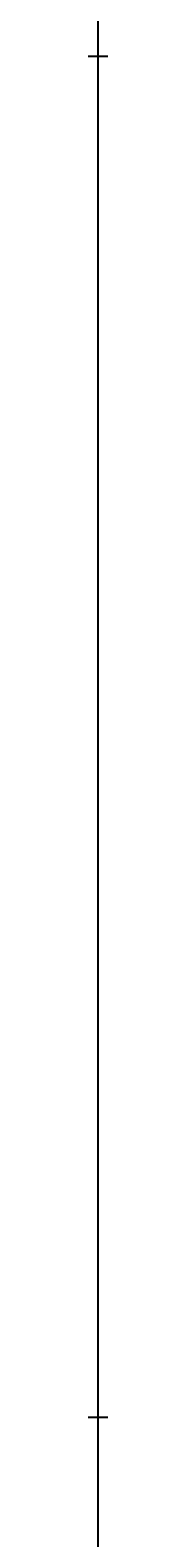
# Model space of a CAD drawing. Units: inches. Extents: x 35362 to 73946, y 43607 to 67532.
# Tile 38 of 134: x 48373 to 48373, y 46091 to 46564. Entities that reach past the tile are written whole.
import ezdxf

# ---------------------------------------------------------------- set-up
doc = ezdxf.new("R2010")
doc.units = ezdxf.units.IN
doc.header["$MEASUREMENT"] = 0
doc.layers.add('A-ANNO-DIMS', color=2, linetype='Continuous', lineweight=18)
doc.styles.get("Standard").update_dxf_attribs({"font": 'arial.ttf'})
doc.dimstyles.get("Standard").update_dxf_attribs({"dimtxt": 0.18, "dimasz": 0.18, "dimexe": 0.18, "dimexo": 0.0625, "dimgap": 0.09, "dimtad": 0, "dimtih": 1, "dimtoh": 1, "dimdec": 4, "dimzin": 0, "dimdsep": 46, "dimtxsty": 'Standard', "dimcen": 0.09, "dimadec": 0, "dimazin": 0, "dimtfac": 1, "dimtdec": 4, "dimtofl": 0, "dimtmove": 0, "dimatfit": 3, "dimfxl": 1, "dimtolj": 1, "dimtzin": 0, "dimarcsym": 0})

# ---------------------------------------------------------------- blocks, each defined once
blk = doc.blocks.new('*D5')
at = {"layer": 'A-ANNO-DIMS', "color": 0, "lineweight": -2, "transparency": 16777216}
for p, q in [((37121.95, 46919.32), (37121.95, 43606.68)), ((69871.5, 45449.83), (69871.5, 43606.68)), ((37122.13, 43606.86), (53496.29, 43606.86)), ((69871.32, 43606.86), (53497.15, 43606.86))]:
    blk.add_line(p, q, dxfattribs=at)
at = {"layer": 'A-ANNO-DIMS', "color": 0, "transparency": 16777216}
for points in [[(37122.13, 43606.89), (37122.13, 43606.83), (37121.95, 43606.86)], [(69871.32, 43606.89), (69871.32, 43606.83), (69871.5, 43606.86)]]:
    blk.add_solid(points, dxfattribs=at)
at = {"layer": 'Defpoints', "color": 0, "transparency": 16777216}
for p in [(37121.95, 46919.38), (69871.5, 45449.89), (69871.5, 43606.86)]:
    blk.add_point(p, dxfattribs=at)
at = {"layer": 'A-ANNO-DIMS', "color": 0, "transparency": 16777216, "insert": (53496.72, 43606.86), "char_height": 0.18, "attachment_point": 5}
blk.add_mtext('\\A1;32750', dxfattribs=at)
blk = doc.blocks.new('*D11')
at = {"layer": 'A-ANNO-DIMS', "color": 0, "lineweight": -2, "transparency": 16777216}
for p, q in [((47978.66, 56028.77), (47978.66, 43606.68)), ((53109.76, 56028.77), (53109.76, 43606.68)), ((47978.84, 43606.86), (50543.87, 43606.86)), ((53109.58, 43606.86), (50544.55, 43606.86))]:
    blk.add_line(p, q, dxfattribs=at)
at = {"layer": 'A-ANNO-DIMS', "color": 0, "transparency": 16777216}
for points in [[(47978.84, 43606.89), (47978.84, 43606.83), (47978.66, 43606.86)], [(53109.58, 43606.89), (53109.58, 43606.83), (53109.76, 43606.86)]]:
    blk.add_solid(points, dxfattribs=at)
at = {"layer": 'Defpoints', "color": 0, "transparency": 16777216}
for p in [(47978.66, 56028.84), (53109.76, 56028.84), (53109.76, 43606.86)]:
    blk.add_point(p, dxfattribs=at)
at = {"layer": 'A-ANNO-DIMS', "color": 0, "transparency": 16777216, "insert": (50544.21, 43606.86), "char_height": 0.18, "attachment_point": 5}
blk.add_mtext('\\A1;5131', dxfattribs=at)
blk = doc.blocks.new('*D13')
at = {"layer": 'A-ANNO-DIMS', "color": 0, "lineweight": -2, "transparency": 16777216}
for p, q in [((48373.49, 51694.02), (48373.49, 43606.68)), ((51029.04, 51694.02), (51029.04, 43606.68)), ((48373.67, 43606.86), (49700.8, 43606.86)), ((51028.86, 43606.86), (49701.73, 43606.86))]:
    blk.add_line(p, q, dxfattribs=at)
at = {"layer": 'A-ANNO-DIMS', "color": 0, "transparency": 16777216}
for points in [[(48373.67, 43606.89), (48373.67, 43606.83), (48373.49, 43606.86)], [(51028.86, 43606.89), (51028.86, 43606.83), (51029.04, 43606.86)]]:
    blk.add_solid(points, dxfattribs=at)
at = {"layer": 'Defpoints', "color": 0, "transparency": 16777216}
for p in [(48373.49, 51694.09), (51029.04, 51694.09), (51029.04, 43606.86)]:
    blk.add_point(p, dxfattribs=at)
at = {"layer": 'A-ANNO-DIMS', "color": 0, "transparency": 16777216, "insert": (49701.27, 43606.86), "char_height": 0.18, "attachment_point": 5}
blk.add_mtext('\\A1;2655.6', dxfattribs=at)
blk = doc.blocks.new('*D67')
at = {"layer": 'A-ANNO-DIMS', "color": 0, "lineweight": -2, "transparency": 16777216}
for p, q in [((56873.54, 53351.53), (35361.77, 53351.53)), ((35361.95, 53351.35), (35361.95, 49400.89)), ((35361.95, 45450.07), (35361.95, 49400.53)), ((53793.58, 45449.89), (35361.77, 45449.89))]:
    blk.add_line(p, q, dxfattribs=at)
at = {"layer": 'A-ANNO-DIMS', "color": 0, "transparency": 16777216}
for points in [[(35361.92, 53351.35), (35361.98, 53351.35), (35361.95, 53351.53)], [(35361.92, 45450.07), (35361.98, 45450.07), (35361.95, 45449.89)]]:
    blk.add_solid(points, dxfattribs=at)
at = {"layer": 'Defpoints', "color": 0, "transparency": 16777216}
for p in [(35361.95, 53351.53), (56873.6, 53351.53), (53793.64, 45449.89)]:
    blk.add_point(p, dxfattribs=at)
at = {"layer": 'A-ANNO-DIMS', "color": 0, "transparency": 16777216, "insert": (35361.95, 49400.71), "char_height": 0.18, "attachment_point": 5}
blk.add_mtext('\\A1;7901.6', dxfattribs=at)
blk = doc.blocks.new('*D76')
at = {"layer": 'A-ANNO-DIMS', "color": 0, "lineweight": -2, "transparency": 16777216}
for p, q in [((54052.84, 46555.29), (35361.77, 46555.29)), ((35361.95, 46555.11), (35361.95, 46342.27)), ((35361.95, 46129.06), (35361.95, 46341.9)), ((53793.58, 46128.88), (35361.77, 46128.88))]:
    blk.add_line(p, q, dxfattribs=at)
at = {"layer": 'A-ANNO-DIMS', "color": 0, "transparency": 16777216}
for points in [[(35361.92, 46555.11), (35361.98, 46555.11), (35361.95, 46555.29)], [(35361.92, 46129.06), (35361.98, 46129.06), (35361.95, 46128.88)]]:
    blk.add_solid(points, dxfattribs=at)
at = {"layer": 'Defpoints', "color": 0, "transparency": 16777216}
for p in [(35361.95, 46555.29), (54052.9, 46555.29), (53793.64, 46128.88)]:
    blk.add_point(p, dxfattribs=at)
at = {"layer": 'A-ANNO-DIMS', "color": 0, "transparency": 16777216, "insert": (35361.95, 46342.09), "char_height": 0.18, "attachment_point": 5}
blk.add_mtext('\\A1;426.4', dxfattribs=at)
blk = doc.blocks.new('*D90')
at = {"layer": 'A-ANNO-DIMS', "color": 0, "lineweight": -2, "transparency": 16777216}
for p, q in [((53707.72, 47291.29), (35361.77, 47291.29)), ((35361.95, 47291.11), (35361.95, 46710.26)), ((35361.95, 46129.06), (35361.95, 46709.9)), ((53793.58, 46128.88), (35361.77, 46128.88))]:
    blk.add_line(p, q, dxfattribs=at)
at = {"layer": 'A-ANNO-DIMS', "color": 0, "transparency": 16777216}
for points in [[(35361.92, 47291.11), (35361.98, 47291.11), (35361.95, 47291.29)], [(35361.92, 46129.06), (35361.98, 46129.06), (35361.95, 46128.88)]]:
    blk.add_solid(points, dxfattribs=at)
at = {"layer": 'Defpoints', "color": 0, "transparency": 16777216}
for p in [(53707.78, 47291.29), (35361.95, 46128.88), (53793.64, 46128.88)]:
    blk.add_point(p, dxfattribs=at)
at = {"layer": 'A-ANNO-DIMS', "color": 0, "transparency": 16777216, "insert": (35361.95, 46710.08), "char_height": 0.18, "attachment_point": 5}
blk.add_mtext('\\A1;1162.4', dxfattribs=at)

msp = doc.modelspace()

# ---------------------------------------------------------------- dimensions: what is measured, and where the dimension line sits
at = {"layer": 'A-ANNO-DIMS'}
for base, p1, p2, override, picture, middle in [((53109.76, 43606.859), (47978.665, 56028.836), (53109.76, 56028.836), {"dimdec": 0, "dimlfac": 1, "dimrnd": 0, "dimzin": 0, "dimdsep": 46, "dimlunit": 2}, '*D11', (50544.212, 43606.859)), ((51029.043, 43606.859), (48373.492, 51694.087), (51029.043, 51694.087), {"dimdec": 1, "dimlfac": 1, "dimrnd": 0, "dimzin": 0, "dimdsep": 46, "dimlunit": 2}, '*D13', (49701.267, 43606.859)), ((69871.496, 43606.859), (37121.949, 46919.381), (69871.496, 45449.894), {"dimdec": 0, "dimlfac": 1, "dimrnd": 0, "dimzin": 0, "dimdsep": 46, "dimlunit": 2}, '*D5', (53496.723, 43606.859))]:
    dim = msp.add_linear_dim(base=base, p1=p1, p2=p2, dimstyle='Standard', override=override, dxfattribs=at)
    dim.commit()
    dim.dimension.update_dxf_attribs({"geometry": picture, "text_midpoint": middle})
for base, p1, p2, picture, middle in [((35361.949, 53351.529), (53793.638, 45449.894), (56873.602, 53351.529), '*D67', (35361.949, 49400.712)), ((35361.949, 46128.878), (53707.781, 47291.285), (53793.638, 46128.878), '*D90', (35361.949, 46710.081)), ((35361.949, 46555.293), (53793.638, 46128.878), (54052.899, 46555.293), '*D76', (35361.949, 46342.086))]:
    dim = msp.add_linear_dim(base=base, p1=p1, p2=p2, angle=90, dimstyle='Standard', override={"dimdec": 1, "dimlfac": 1, "dimrnd": 0, "dimzin": 0, "dimdsep": 46, "dimlunit": 2}, dxfattribs=at)
    dim.commit()
    dim.dimension.update_dxf_attribs({"geometry": picture, "text_midpoint": middle})

doc.saveas('drawing.dxf')
